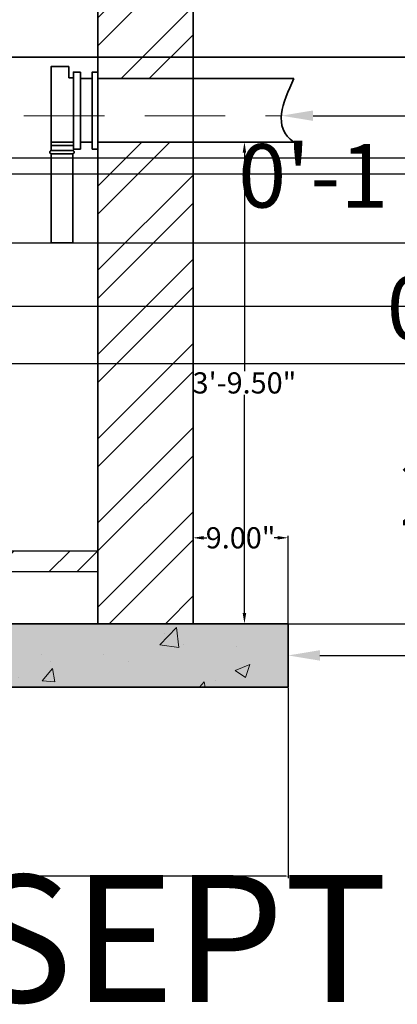
# Model space of a CAD drawing. Units: inches. Extents: x -34 to 285, y -151 to 155.
# Tile 7 of 10: x 189 to 225, y -151 to -58. Entities that reach past the tile are written whole.
import ezdxf
from ezdxf import colors
from ezdxf.entities.mleader import LeaderData, LeaderLine
from ezdxf.math import Vec2, Vec3

# ---------------------------------------------------------------- set-up
doc = ezdxf.new("R2010")
doc.units = ezdxf.units.IN
doc.header["$MEASUREMENT"] = 0
doc.linetypes.add('DASHED', pattern=[19.05, 12.7, -6.35])
for name, color, linetype, lineweight in [('A-ANNO-DIMS', 2, 'Continuous', 18), ('A-ANNO-TEXT', 7, 'Continuous', 25), ('A-DETL', 7, 'Continuous', 35), ('A-DETL-HIDN', 8, 'DASHED', 18), ('A-DETL-PATT', 8, 'Continuous', 18), ('A-FLOR-STRS', 3, 'Continuous', 25), ('P-SANR-PATT', 8, 'Continuous', 13), ('P-SANR-PIPE', 4, 'Continuous', 35)]:
    doc.layers.add(name, color=color, linetype=linetype, lineweight=lineweight)
doc.styles.get("Standard").update_dxf_attribs({"font": 'arial.ttf'})
doc.dimstyles.get("Standard").update_dxf_attribs({"dimtxt": 6, "dimasz": 0.18, "dimexe": 0.18, "dimexo": 0.0625, "dimgap": 0.09, "dimtad": 0, "dimtih": 1, "dimtoh": 1, "dimzin": 0, "dimdsep": 46, "dimlunit": 3, "dimtxsty": 'Standard', "dimcen": 0.09, "dimadec": 0, "dimazin": 0, "dimtfac": 1, "dimtofl": 0, "dimtmove": 0, "dimatfit": 3, "dimfxl": 1, "dimtolj": 1, "dimtzin": 0, "dimarcsym": 0})

# ---------------------------------------------------------------- blocks, each defined once
blk = doc.blocks.new('*D30')
at = {"layer": 'A-ANNO-DIMS', "color": 0, "lineweight": -2, "transparency": 16777216}
for p, q in [((205.908, -69.469), (210.892, -69.469)), ((210.712, -70.469), (210.712, -91.107)), ((210.712, -113.969), (210.712, -93.331)), ((205.908, -114.969), (210.892, -114.969))]:
    blk.add_line(p, q, dxfattribs=at)
at = {"layer": 'A-ANNO-DIMS', "color": 0, "transparency": 16777216}
for points in [[(210.545, -70.469), (210.878, -70.469), (210.712, -69.469)], [(210.545, -113.969), (210.878, -113.969), (210.712, -114.969)]]:
    blk.add_solid(points, dxfattribs=at)
at = {"layer": 'Defpoints', "color": 0, "transparency": 16777216}
for p in [(205.846, -69.469), (205.846, -114.969), (210.712, -114.969)]:
    blk.add_point(p, dxfattribs=at)
at = {"layer": 'A-ANNO-DIMS', "color": 0, "transparency": 16777216, "insert": (210.712, -92.219), "char_height": 2, "attachment_point": 5}
blk.add_mtext('\\A1;3\'-9.50"', dxfattribs=at)
blk = doc.blocks.new('*D31')
at = {"layer": 'A-ANNO-DIMS', "color": 0, "lineweight": -2, "transparency": 16777216}
for p, q in [((205.846, -114.906), (205.846, -106.675)), ((206.846, -106.855), (207.164, -106.855)), ((213.846, -106.855), (213.527, -106.855)), ((214.846, -114.906), (214.846, -106.675))]:
    blk.add_line(p, q, dxfattribs=at)
at = {"layer": 'A-ANNO-DIMS', "color": 0, "transparency": 16777216}
for points in [[(206.846, -106.688), (206.846, -107.022), (205.846, -106.855)], [(213.846, -106.688), (213.846, -107.022), (214.846, -106.855)]]:
    blk.add_solid(points, dxfattribs=at)
at = {"layer": 'Defpoints', "color": 0, "transparency": 16777216}
for p in [(214.846, -106.855), (205.846, -114.969), (214.846, -114.969)]:
    blk.add_point(p, dxfattribs=at)
at = {"layer": 'A-ANNO-DIMS', "color": 0, "transparency": 16777216, "insert": (210.346, -106.855), "char_height": 2, "attachment_point": 5}
blk.add_mtext('\\A1;9.00"', dxfattribs=at)
blk = doc.blocks.new('PIPE-SOCKET')
for p, q in [((1.802, 8.25), (0.129, 8.25)), ((1.802, 7.168), (1.802, 8.25)), ((2.233, 7.168), (1.802, 7.168)), ((2.233, 7.168), (2.233, 7.168))]:
    blk.add_line(p, q)
for points in [[(0.129, 0.312), (0.129, 8.25), (1.802, 8.25)], [(0.129, 0.312), (2.172, 0.312)]]:
    blk.add_lwpolyline(points)
for centre, start, end in [((0.157, 0.157), 100.54101, 280.54101), ((2.144, 0.157), 259.45899, 79.45899)]:
    blk.add_arc(centre, 0.157, start, end)
blk = doc.blocks.new('*D48')
at = {"layer": 'A-ANNO-DIMS', "color": 0, "lineweight": -2, "transparency": 16777216}
for p, q in [((22.846, -121.031), (22.846, -138.999)), ((214.846, -121.031), (214.846, -138.999)), ((23.026, -138.819), (108.733, -138.819)), ((214.666, -138.819), (128.959, -138.819))]:
    blk.add_line(p, q, dxfattribs=at)
at = {"layer": 'A-ANNO-DIMS', "color": 0, "transparency": 16777216}
for points in [[(23.026, -138.789), (23.026, -138.849), (22.846, -138.819)], [(214.666, -138.789), (214.666, -138.849), (214.846, -138.819)]]:
    blk.add_solid(points, dxfattribs=at)
at = {"layer": 'Defpoints', "color": 0, "transparency": 16777216}
for p in [(22.846, -120.969), (214.846, -120.969), (214.846, -138.819)]:
    blk.add_point(p, dxfattribs=at)
at = {"layer": 'A-ANNO-DIMS', "color": 0, "transparency": 16777216, "insert": (118.846, -138.819), "char_height": 6, "attachment_point": 5}
blk.add_mtext('\\A1;16\'-0"', dxfattribs=at)
blk = doc.blocks.new('*D59')
at = {"layer": 'A-ANNO-DIMS', "color": 0, "lineweight": -2, "transparency": 16777216}
for p, q in [((83.148, -48.969), (241.637, -48.969)), ((241.457, -49.149), (241.457, -52)), ((241.457, -61.235), (241.457, -58.384)), ((89.009, -61.415), (241.637, -61.415))]:
    blk.add_line(p, q, dxfattribs=at)
at = {"layer": 'A-ANNO-DIMS', "color": 0, "transparency": 16777216}
for points in [[(241.427, -49.149), (241.487, -49.149), (241.457, -48.969)], [(241.427, -61.235), (241.487, -61.235), (241.457, -61.415)]]:
    blk.add_solid(points, dxfattribs=at)
at = {"layer": 'Defpoints', "color": 0, "transparency": 16777216}
for p in [(83.086, -48.969), (88.947, -61.415), (241.457, -61.415)]:
    blk.add_point(p, dxfattribs=at)
at = {"layer": 'A-ANNO-DIMS', "color": 0, "transparency": 16777216, "insert": (241.457, -55.192), "char_height": 6, "attachment_point": 5}
blk.add_mtext('\\A1;1\'-0 1/2"', dxfattribs=at)
blk = doc.blocks.new('*D62')
at = {"layer": 'A-ANNO-DIMS', "color": 0, "lineweight": -2, "transparency": 16777216}
for p, q in [((155.218, -48.969), (241.637, -48.969)), ((241.457, -49.149), (241.457, -52.018)), ((241.457, -61.271), (241.457, -58.402)), ((153.777, -61.451), (241.637, -61.451))]:
    blk.add_line(p, q, dxfattribs=at)
at = {"layer": 'A-ANNO-DIMS', "color": 0, "transparency": 16777216}
for points in [[(241.427, -49.149), (241.487, -49.149), (241.457, -48.969)], [(241.427, -61.271), (241.487, -61.271), (241.457, -61.451)]]:
    blk.add_solid(points, dxfattribs=at)
at = {"layer": 'Defpoints', "color": 0, "transparency": 16777216}
for p in [(155.156, -48.969), (153.715, -61.451), (241.457, -61.451)]:
    blk.add_point(p, dxfattribs=at)
at = {"layer": 'A-ANNO-DIMS', "color": 0, "transparency": 16777216, "insert": (241.457, -55.21), "char_height": 6, "attachment_point": 5}
blk.add_mtext('\\A1;1\'-0 1/2"', dxfattribs=at)
blk = doc.blocks.new('*D65')
at = {"layer": 'A-ANNO-DIMS', "color": 0, "lineweight": -2, "transparency": 16777216}
for p, q in [((130.158, -90.369), (241.637, -90.369)), ((241.457, -90.549), (241.457, -99.477)), ((241.457, -114.789), (241.457, -105.861)), ((139.908, -114.969), (241.637, -114.969))]:
    blk.add_line(p, q, dxfattribs=at)
at = {"layer": 'A-ANNO-DIMS', "color": 0, "transparency": 16777216}
for points in [[(241.427, -90.549), (241.487, -90.549), (241.457, -90.369)], [(241.427, -114.789), (241.487, -114.789), (241.457, -114.969)]]:
    blk.add_solid(points, dxfattribs=at)
at = {"layer": 'Defpoints', "color": 0, "transparency": 16777216}
for p in [(130.096, -90.369), (139.846, -114.969), (241.457, -114.969)]:
    blk.add_point(p, dxfattribs=at)
at = {"layer": 'A-ANNO-DIMS', "color": 0, "transparency": 16777216, "insert": (241.457, -102.669), "char_height": 6, "attachment_point": 5}
blk.add_mtext('\\A1;2\'-0 1/2"', dxfattribs=at)
blk = doc.blocks.new('*D66')
at = {"layer": 'A-ANNO-DIMS', "color": 0, "lineweight": -2, "transparency": 16777216}
for p, q in [((157.908, -78.969), (241.637, -78.969)), ((241.457, -79.149), (241.457, -84.789)), ((157.908, -84.969), (241.637, -84.969)), ((241.457, -85.149), (241.277, -85.149)), ((241.457, -84.969), (241.457, -85.149))]:
    blk.add_line(p, q, dxfattribs=at)
at = {"layer": 'A-ANNO-DIMS', "color": 0, "transparency": 16777216}
for points in [[(241.427, -79.149), (241.487, -79.149), (241.457, -78.969)], [(241.427, -84.789), (241.487, -84.789), (241.457, -84.969)]]:
    blk.add_solid(points, dxfattribs=at)
at = {"layer": 'Defpoints', "color": 0, "transparency": 16777216}
for p in [(157.846, -78.969), (157.846, -84.969), (241.457, -84.969)]:
    blk.add_point(p, dxfattribs=at)
at = {"layer": 'A-ANNO-DIMS', "color": 0, "transparency": 16777216, "insert": (233.213, -85.149), "char_height": 6, "attachment_point": 5}
blk.add_mtext('\\A1;0\'-6"', dxfattribs=at)
blk = doc.blocks.new('*D78')
at = {"layer": 'A-ANNO-DIMS', "color": 0, "lineweight": -2, "transparency": 16777216}
for p, q in [((96.293, -70.947), (241.637, -70.947)), ((241.457, -71.127), (241.457, -72.29)), ((96.293, -72.47), (241.637, -72.47)), ((241.457, -72.47), (241.457, -72.65)), ((241.457, -72.65), (241.277, -72.65))]:
    blk.add_line(p, q, dxfattribs=at)
at = {"layer": 'A-ANNO-DIMS', "color": 0, "transparency": 16777216}
for points in [[(241.427, -71.127), (241.487, -71.127), (241.457, -70.947)], [(241.427, -72.29), (241.487, -72.29), (241.457, -72.47)]]:
    blk.add_solid(points, dxfattribs=at)
at = {"layer": 'Defpoints', "color": 0, "transparency": 16777216}
for p in [(96.231, -70.947), (96.231, -72.47), (241.457, -72.47)]:
    blk.add_point(p, dxfattribs=at)
at = {"layer": 'A-ANNO-DIMS', "color": 0, "transparency": 16777216, "insert": (226.222, -72.65), "char_height": 6, "attachment_point": 5}
blk.add_mtext('\\A1;0\'-1 1/2"', dxfattribs=at)
blk = doc.blocks.new('*D80')
at = {"layer": 'A-ANNO-DIMS', "color": 0, "lineweight": -2, "transparency": 16777216}
for p, q in [((162.715, -73.74), (162.715, -18.978)), ((162.895, -19.158), (169.123, -19.158)), ((169.303, -84.63), (169.303, -18.978)), ((169.303, -19.158), (169.483, -19.158))]:
    blk.add_line(p, q, dxfattribs=at)
at = {"layer": 'A-ANNO-DIMS', "color": 0, "transparency": 16777216}
for points in [[(162.895, -19.128), (162.895, -19.188), (162.715, -19.158)], [(169.123, -19.128), (169.123, -19.188), (169.303, -19.158)]]:
    blk.add_solid(points, dxfattribs=at)
at = {"layer": 'Defpoints', "color": 0, "transparency": 16777216}
for p in [(169.303, -19.158), (162.715, -73.803), (169.303, -84.693)]:
    blk.add_point(p, dxfattribs=at)
at = {"layer": 'A-ANNO-DIMS', "color": 0, "transparency": 16777216, "insert": (184.538, -19.158), "char_height": 6, "attachment_point": 5}
blk.add_mtext('\\A1;0\'-6 1/2"', dxfattribs=at)
blk = doc.blocks.new('*D81')
at = {"layer": 'A-ANNO-DIMS', "color": 0, "lineweight": -2, "transparency": 16777216}
for p, q in [((169.303, -84.63), (169.303, -18.978)), ((169.483, -19.158), (179.302, -19.158)), ((179.482, -96.63), (179.482, -18.978)), ((179.482, -19.158), (179.662, -19.158))]:
    blk.add_line(p, q, dxfattribs=at)
at = {"layer": 'A-ANNO-DIMS', "color": 0, "transparency": 16777216}
for points in [[(169.483, -19.128), (169.483, -19.188), (169.303, -19.158)], [(179.302, -19.128), (179.302, -19.188), (179.482, -19.158)]]:
    blk.add_solid(points, dxfattribs=at)
at = {"layer": 'Defpoints', "color": 0, "transparency": 16777216}
for p in [(179.482, -19.158), (169.303, -84.693), (179.482, -96.693)]:
    blk.add_point(p, dxfattribs=at)
at = {"layer": 'A-ANNO-DIMS', "color": 0, "transparency": 16777216, "insert": (190.057, -19.158), "char_height": 6, "attachment_point": 5}
blk.add_mtext('\\A1;0\'-10"', dxfattribs=at)
blk = doc.blocks.new('*D82')
at = {"layer": 'A-ANNO-DIMS', "color": 0, "lineweight": -2, "transparency": 16777216}
for p, q in [((179.482, -96.63), (179.482, -18.978)), ((179.662, -19.158), (187.666, -19.158)), ((187.846, -108.007), (187.846, -18.978)), ((187.846, -19.158), (188.026, -19.158))]:
    blk.add_line(p, q, dxfattribs=at)
at = {"layer": 'A-ANNO-DIMS', "color": 0, "transparency": 16777216}
for points in [[(179.662, -19.128), (179.662, -19.188), (179.482, -19.158)], [(187.666, -19.128), (187.666, -19.188), (187.846, -19.158)]]:
    blk.add_solid(points, dxfattribs=at)
at = {"layer": 'Defpoints', "color": 0, "transparency": 16777216}
for p in [(187.846, -19.158), (179.482, -96.693), (187.846, -108.07)]:
    blk.add_point(p, dxfattribs=at)
at = {"layer": 'A-ANNO-DIMS', "color": 0, "transparency": 16777216, "insert": (203.081, -19.158), "char_height": 6, "attachment_point": 5}
blk.add_mtext('\\A1;0\'-8 1/2"', dxfattribs=at)
blk = doc.blocks.new('*D87')
at = {"layer": 'A-ANNO-DIMS', "color": 0, "lineweight": -2, "transparency": 16777216}
for p, q in [((187.783, -108.07), (0.722, -108.07)), ((0.902, -108.25), (0.902, -108.366)), ((196.783, -114.969), (0.722, -114.969)), ((0.902, -114.789), (0.902, -114.673))]:
    blk.add_line(p, q, dxfattribs=at)
at = {"layer": 'A-ANNO-DIMS', "color": 0, "transparency": 16777216}
for points in [[(0.872, -108.25), (0.932, -108.25), (0.902, -108.07)], [(0.872, -114.789), (0.932, -114.789), (0.902, -114.969)]]:
    blk.add_solid(points, dxfattribs=at)
at = {"layer": 'Defpoints', "color": 0, "transparency": 16777216}
for p in [(187.846, -108.07), (0.902, -114.969), (196.846, -114.969)]:
    blk.add_point(p, dxfattribs=at)
at = {"layer": 'A-ANNO-DIMS', "color": 0, "transparency": 16777216, "insert": (0.902, -111.519), "char_height": 6, "attachment_point": 5}
blk.add_mtext('\\A1;0\'-7"', dxfattribs=at)

msp = doc.modelspace()

# ---------------------------------------------------------------- hatches: boundary and pattern name
at = {"layer": 'A-DETL-PATT'}
h = msp.add_hatch(dxfattribs=at)
h.set_pattern_fill('AR-CONC', color=256, scale=0.4)
h.set_pattern_definition([(50, (0, 0), (2.86904, -0.251009), [0.3, -3.3]), (355, (0, 0), (-0.555005, 3.00877), [0.24, -2.64]), (100.4514, (0.239, -0.021), (2.314035, 2.75776), [0.25496, -2.80457]), (46.1842, (0, 0.8), (4.268965, -0.662077), [0.45, -4.95]), (96.6356, (0.3557, 0.745), (3.73865, 3.896474), [0.38244, -4.206855]), (351.1842, (0, 0.8), (3.73865, 3.896474), [0.36, -3.96]), (21, (0.4, 0.6), (2.387628, -1.610476), [0.3, -3.3]), (326, (0.4, 0.6), (0.97326, 2.9006), [0.24, -2.64]), (71.4514, (0.599, 0.4658), (3.36089, 1.290125), [0.25496, -2.80457]), (37.5, (0, 0), (0.0486394, 1.3315754), [0, -2.608, 0, -2.68, 0, -2.65]), (7.5, (0, 0), (1.052278, 1.577647), [0, -1.528, 0, -2.548, 0, -1.01]), (327.5, (-0.892, 0), (2.1352897, -0.0902195), [0, -1, 0, -3.12, 0, -4.14]), (317.5, (-1.292, 0), (2.332745, 0.40042), [0, -1.3, 0, -2.072, 0, -2.94])])
h.paths.add_polyline_path([(214.846, -48.969), (214.846, -42.969), (184.518, -42.969), (184.518, -48.969)])
h.paths.add_polyline_path([(122.241, -42.969), (122.241, -48.969), (155.156, -48.969), (155.156, -42.969)])
h.paths.add_polyline_path([(214.846, -114.969), (22.846, -114.969), (22.846, -120.969), (214.846, -120.969)])
h = msp.add_hatch(dxfattribs=at)
h.set_pattern_fill('ANSI32', color=256, scale=15)
h.paths.add_polyline_path([(205.846, -48.969), (196.846, -48.969), (196.846, -63.469), (205.846, -63.469)])
h = msp.add_hatch(dxfattribs=at)
h.set_pattern_fill('ANSI32', color=256, scale=15)
h.paths.add_polyline_path([(171.715, -73.803), (162.715, -73.803), (162.715, -75.803), (171.715, -75.803)])
h.paths.add_polyline_path([(178.303, -84.693), (169.303, -84.693), (169.303, -86.693), (178.303, -86.693)])
h.paths.add_polyline_path([(188.482, -96.693), (179.482, -96.693), (179.482, -98.693), (188.482, -98.693)])
h.paths.add_polyline_path([(196.846, -108.07), (187.846, -108.07), (187.846, -110.07), (196.846, -110.07)])
h.paths.add_polyline_path([(162.715, -61.451), (153.715, -61.451), (153.715, -63.451), (162.715, -63.451)])
h = msp.add_hatch(dxfattribs=at)
h.set_pattern_fill('ANSI32', color=256, scale=15)
h.paths.add_polyline_path([(205.846, -69.469), (196.846, -69.469), (196.846, -70.12), (196.846, -114.969), (205.846, -114.969)])
h = msp.add_hatch(dxfattribs=at)
h.set_pattern_fill('AR-CONC', color=256, scale=2)
h.paths.add_polyline_path([(22.846, -114.969), (22.846, -120.969), (214.846, -120.969), (214.846, -114.969)])
at = {"layer": 'P-SANR-PATT'}
h = msp.add_hatch(dxfattribs=at)
h.set_pattern_fill('AR-CONC', color=256, scale=2)
h.paths.add_polyline_path([(196.846, -62.851), (196.308, -62.851), (196.308, -70.12), (196.846, -70.12)])
h.paths.add_polyline_path([(195.189, -62.851), (194.536, -62.851), (194.536, -70.12), (195.189, -70.12)])
h = msp.add_hatch(dxfattribs=at)
h.set_pattern_fill('AR-CONC', color=256, scale=2)
h.paths.add_polyline_path([(194.536, -69.469), (192.432, -69.469), (192.432, -69.778), (194.536, -69.778)])
h = msp.add_hatch(dxfattribs=at)
h.set_pattern_fill('AR-CONC', color=256, scale=2)
h.paths.add_polyline_path([(194.475, -70.255), (192.432, -70.255, 0.831086), (192.432, -70.564), (194.475, -70.564, 0.831086)])

# ---------------------------------------------------------------- linework, layer by layer
at = {"layer": 'A-DETL'}
for p, q in [((196.846, -48.969), (196.846, -114.969)), ((205.846, -48.969), (205.846, -114.969)), ((22.846, -114.969), (214.846, -114.969)), ((214.846, -114.969), (214.846, -120.969)), ((22.846, -120.969), (214.846, -120.969))]:
    msp.add_line(p, q, dxfattribs=at)
at = {"layer": 'A-DETL-HIDN', "ltscale": 0.6}
msp.add_line((75.547, -66.969), (214.207, -66.969), dxfattribs=at)
at = {"layer": 'A-FLOR-STRS'}
msp.add_lwpolyline([(196.846, -110.07), (187.846, -110.07), (187.846, -108.07), (196.846, -108.07)], close=True, dxfattribs=at)
at = {"layer": 'P-SANR-PIPE'}
for p, q in [((196.846, -63.469), (215.397, -63.469)), ((196.846, -63.469), (205.846, -63.469)), ((195.189, -69.469), (196.308, -69.469)), ((196.846, -69.469), (215.397, -69.469)), ((196.846, -69.469), (205.846, -69.469)), ((196.846, -69.469), (214.846, -69.469)), ((192.432, -78.969), (194.475, -78.969))]:
    msp.add_line(p, q, dxfattribs=at)
for points in [[(195.189, -62.851), (194.536, -62.851), (194.536, -70.12), (195.189, -70.12)], [(196.846, -62.851), (196.308, -62.851), (196.308, -70.12), (196.846, -70.12)], [(196.308, -63.469), (195.189, -63.469), (195.189, -69.469), (196.308, -69.469)]]:
    msp.add_lwpolyline(points, close=True, dxfattribs=at)
for points in [[(215.397, -69.469), (205.846, -69.469), (205.846, -63.469), (215.397, -63.469)], [(194.536, -69.778), (192.432, -69.778), (192.432, -69.469), (194.475, -69.469)], [(194.475, -70.564), (192.432, -70.564)], [(194.475, -70.564), (194.475, -78.969), (192.432, -78.969), (192.432, -70.564)]]:
    msp.add_lwpolyline(points, dxfattribs=at)
msp.add_open_spline([(215.397, -63.469), (214.356, -65.755), (213.314, -68.04), (215.397, -69.469)], degree=3, dxfattribs=at)

# ---------------------------------------------------------------- block references
msp.add_blockref('PIPE-SOCKET', (192.303, -70.567), dxfattribs=at)

# ---------------------------------------------------------------- texts
at = {"layer": 'A-ANNO-TEXT', "insert": (-34.52, -138.72), "char_height": 12, "attachment_point": 1}
msp.add_mtext_dynamic_manual_height_columns('SECTIONAL ELEVATION OF A SEPTIC TANK ', width=509.35271, gutter_width=1, heights=[0], dxfattribs=at)

# ---------------------------------------------------------------- dimensions: what is measured, and where the dimension line sits
at = {"layer": 'A-ANNO-DIMS'}
for base, p1, p2, override, picture, middle in [((169.303, -19.158), (162.715, -73.803), (169.303, -84.693), {"dimdec": 1, "dimlfac": 1, "dimrnd": 0, "dimzin": 1, "dimdsep": 46, "dimlunit": 4, "dimfrac": 2}, '*D80', (184.538, -19.158)), ((187.846, -19.158), (179.482, -96.693), (187.846, -108.07), {"dimdec": 1, "dimlfac": 1, "dimrnd": 0, "dimzin": 1, "dimdsep": 46, "dimlunit": 4, "dimfrac": 2}, '*D82', (203.081, -19.158)), ((179.482, -19.158), (169.303, -84.693), (179.482, -96.693), {"dimdec": 1, "dimlfac": 1, "dimrnd": 0, "dimzin": 1, "dimdsep": 46, "dimlunit": 4, "dimfrac": 2}, '*D81', (190.057, -19.158)), ((214.846, -106.855), (205.846, -114.969), (214.846, -114.969), {"dimtxt": 2, "dimasz": 1, "dimclrd": 0, "dimclre": 0, "dimclrt": 0}, '*D31', (210.346, -106.855)), ((214.846, -138.819), (22.846, -120.969), (214.846, -120.969), {"dimdec": 1, "dimlfac": 1, "dimrnd": 0, "dimzin": 1, "dimdsep": 46, "dimlunit": 4, "dimfrac": 2}, '*D48', (118.846, -138.819))]:
    dim = msp.add_linear_dim(base=base, p1=p1, p2=p2, dimstyle='Standard', override=override, dxfattribs=at)
    dim.commit()
    dim.dimension.update_dxf_attribs({"geometry": picture, "text_midpoint": middle})
for base, p1, p2, override, picture, middle in [((241.457, -61.415), (83.086, -48.969), (88.947, -61.415), {"dimdec": 1, "dimlfac": 1, "dimrnd": 0, "dimzin": 1, "dimdsep": 46, "dimlunit": 4, "dimfrac": 2}, '*D59', (241.457, -55.192)), ((241.457, -61.451), (155.156, -48.969), (153.715, -61.451), {"dimdec": 1, "dimlfac": 1, "dimrnd": 0, "dimzin": 1, "dimdsep": 46, "dimlunit": 4, "dimfrac": 2}, '*D62', (241.457, -55.21)), ((241.457, -72.47), (96.231, -70.947), (96.231, -72.47), {"dimdec": 1, "dimlfac": 1, "dimrnd": 0, "dimzin": 1, "dimdsep": 46, "dimlunit": 4, "dimfrac": 2}, '*D78', (226.222, -72.65)), ((210.712, -114.969), (205.846, -69.469), (205.846, -114.969), {"dimtxt": 2, "dimasz": 1, "dimclrd": 0, "dimclre": 0, "dimclrt": 0}, '*D30', (210.712, -92.219)), ((241.457, -84.969), (157.846, -78.969), (157.846, -84.969), {"dimdec": 1, "dimlfac": 1, "dimrnd": 0, "dimzin": 1, "dimdsep": 46, "dimlunit": 4, "dimfrac": 2}, '*D66', (233.213, -85.149)), ((241.457, -114.969), (130.096, -90.369), (139.846, -114.969), {"dimdec": 1, "dimlfac": 1, "dimrnd": 0, "dimzin": 1, "dimdsep": 46, "dimlunit": 4, "dimfrac": 2}, '*D65', (241.457, -102.669)), ((0.902, -114.969), (187.846, -108.07), (196.846, -114.969), {"dimdec": 1, "dimlfac": 1, "dimrnd": 0, "dimzin": 1, "dimdsep": 46, "dimlunit": 4, "dimfrac": 2}, '*D87', (0.902, -111.519))]:
    dim = msp.add_linear_dim(base=base, p1=p1, p2=p2, angle=90, dimstyle='Standard', override=override, dxfattribs=at)
    dim.commit()
    dim.dimension.update_dxf_attribs({"geometry": picture, "text_midpoint": middle})

# ---------------------------------------------------------------- leaders
at = {"layer": 'A-ANNO-TEXT'}
ml = msp.add_multileader_mtext('Standard', dxfattribs=at)
ml.set_content('9" THICK BRICK \\PMASONRY ', color=(248, 215, 49))
ml.set_leader_properties()
ml.build(insert=Vec2(0, 0))
ml.multileader.update_dxf_attribs({"dogleg_length": 4.22, "arrow_head_size": 3})
ctx = ml.context
ctx.base_point, ctx.char_height, ctx.arrow_head_size, ctx.landing_gap_size, ctx.plane_origin = Vec3(224.277, -54.411), 1, 3, 0.09, Vec3(205.846, -54.411)
notes = []
notes.append((ctx, [(0, (1, 1, 0), (220.057, -54.411), (1, 0), 4.22, [(0, [(205.846, -54.411)], 0, [])])]))
ctx.mtext.insert, ctx.mtext.flow_direction = Vec3(224.367, -53.902), 5
ml = msp.add_multileader_mtext('Standard', dxfattribs=at)
ml.set_content('OUTLET\\P04" PIPE', color=(248, 215, 49))
ml.set_leader_properties()
ml.build(insert=Vec2(0, 0))
ml.multileader.update_dxf_attribs({"dogleg_length": 4.22, "arrow_head_size": 3})
ctx = ml.context
ctx.base_point, ctx.char_height, ctx.arrow_head_size, ctx.landing_gap_size, ctx.plane_origin = Vec3(234.182, -66.969), 1, 3, 0.09, Vec3(214.207, -66.969)
notes.append((ctx, [(0, (1, 1, 0), (229.962, -66.969), (1, 0), 4.22, [(0, [(214.207, -66.969)], 0, [])])]))
ctx.mtext.insert, ctx.mtext.flow_direction = Vec3(234.272, -66.46), 5
ml = msp.add_multileader_mtext('Standard', dxfattribs=at)
ml.set_content('6" THICK P.C.C ', color=(248, 215, 49))
ml.set_leader_properties()
ml.build(insert=Vec2(0, 0))
ml.multileader.update_dxf_attribs({"dogleg_length": 4.22, "arrow_head_size": 3})
ctx = ml.context
ctx.base_point, ctx.char_height, ctx.arrow_head_size, ctx.landing_gap_size, ctx.plane_origin = Vec3(231.808, -117.969), 1, 3, 0.09, Vec3(214.846, -117.969)
notes.append((ctx, [(0, (1, 1, 0), (227.588, -117.969), (1, 0), 4.22, [(0, [(214.846, -117.969)], 0, [])])]))
ctx.mtext.insert, ctx.mtext.flow_direction = Vec3(231.898, -117.46), 5
for ctx, leaders in notes:
    for number, flags, end, landing, length, lines in leaders:
        leader = LeaderData()
        leader.index, (leader.has_last_leader_line, leader.has_dogleg_vector, leader.attachment_direction) = number, flags
        leader.last_leader_point, leader.dogleg_vector, leader.dogleg_length = Vec3(end), Vec3(landing), length
        for number, points, colour, breaks in lines:
            line = LeaderLine()
            line.index, line.vertices, line.color, line.breaks = number, Vec3.list(points), colors.encode_raw_color(colour), breaks
            leader.lines.append(line)
        ctx.leaders.append(leader)

doc.saveas('drawing.dxf')
